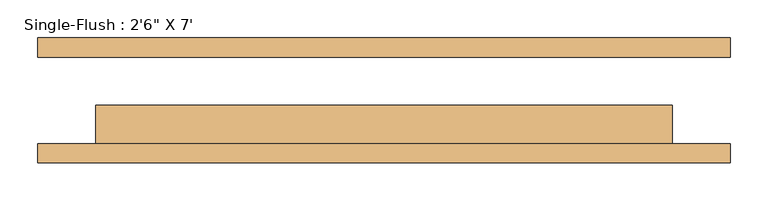
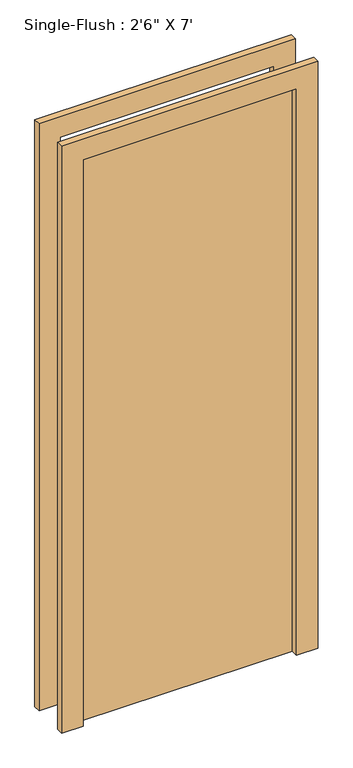
"""IFC4 building model written with IfcOpenShell, lengths in millimetres: door geometry."""

from ifc_helpers import new_model, si_unit, frame, origin, origin_with_axes, place, context, project, spatial, polyline, outline, extrude, source, transform, mapped, element, save


def door_78caadf7(model_context):
    return source(origin(), model_context, "Body", "SweptSolid", [
        extrude(outline(polyline([(2209.8, -457.2), (0.0, -457.2), (0.0, -381.0), (2133.6, -381.0), (2133.6, 381.0), (0.0, 381.0), (0.0, 457.2), (2209.8, 457.2), (2209.8, -457.2)])), frame((0.0, -82.55, 0.0), z_axis=(0.0, 1.0, 0.0), x_axis=(0.0, 0.0, 1.0)), (0.0, 0.0, 1.0), 25.4),
        extrude(outline(polyline([(2209.8, 457.2), (2209.8, -457.2), (0.0, -457.2), (0.0, -381.0), (2133.6, -381.0), (2133.6, 381.0), (0.0, 381.0), (0.0, 457.2), (2209.8, 457.2)])), frame((0.0, 57.15, 0.0), z_axis=(0.0, 1.0, 0.0), x_axis=(0.0, 0.0, 1.0)), (0.0, 0.0, 1.0), 25.4),
        extrude(outline(polyline([(381.0, -6.35), (381.0, -57.15), (-381.0, -57.15), (-381.0, -6.35), (381.0, -6.35)])), origin_with_axes(), (0.0, 0.0, 1.0), 2133.6),
    ])


if __name__ == "__main__":
    model = new_model("IFC4")
    model_context = context("Model", 3, world=origin())
    ifc_project = project(units=[si_unit("LENGTHUNIT", "METRE", prefix="MILLI")], contexts=[model_context])
    site = spatial("IfcSite", under=ifc_project)
    building = spatial("IfcBuilding", under=site)
    placement = place(None, origin())
    door_shape = door_78caadf7(model_context)
    element("IfcDoor", 1, ObjectType="Single-Flush : 2'6\" X 7'", at=placement, inside=building, context=model_context, shape_type="MappedRepresentation", body=[
        mapped(door_shape, transform((0.0, 0.0, 0.0), x_axis=(1.0, 0.0, 0.0), y_axis=(0.0, 1.0, 0.0), z_axis=(0.0, 0.0, 1.0))),
    ])
    save(model, "model.ifc")

# Revit data of these elements
# Type "Single-Flush : 2'6\" X 7'"
#   Type Mark = "14"
#   Construction Type Id = "MDOOR"
#   Assembly Code = "C1020"
#   Analytic Construction = "Metal"
#   Thickness = 0' - 2"
#   Heat Transfer Coefficient (U) = 0.651978 BTU/(h·ft²·°F)
#   Height = 7' - 0"
#   Trim Projection Ext = 0' - 1"
#   Trim Projection Int = 0' - 1"
#   Trim Width = 0' - 3"
#   Width = 2' - 6"
#   Define Thermal Properties by = 1
#   Door Material = Door - Panel
#   Frame Material = Door - Frame
#   Visual Light Transmittance = 0
#   Solar Heat Gain Coefficient = 0
#   Function = (empty or 0)
#   Wall Closure = (empty or 0)
# Element 1 (IfcDoor, "Single-Flush : 2'6\" X 7'")
#   Materials on its faces: "Door - Frame", "Door - Panel"
# Materials
#   "Door - Panel": class "Wood", colour RGB 210 159 95, transparency 0, Cost = 0
#   "Door - Frame": colour RGB 118 70 51, transparency 0, Cost = 0
